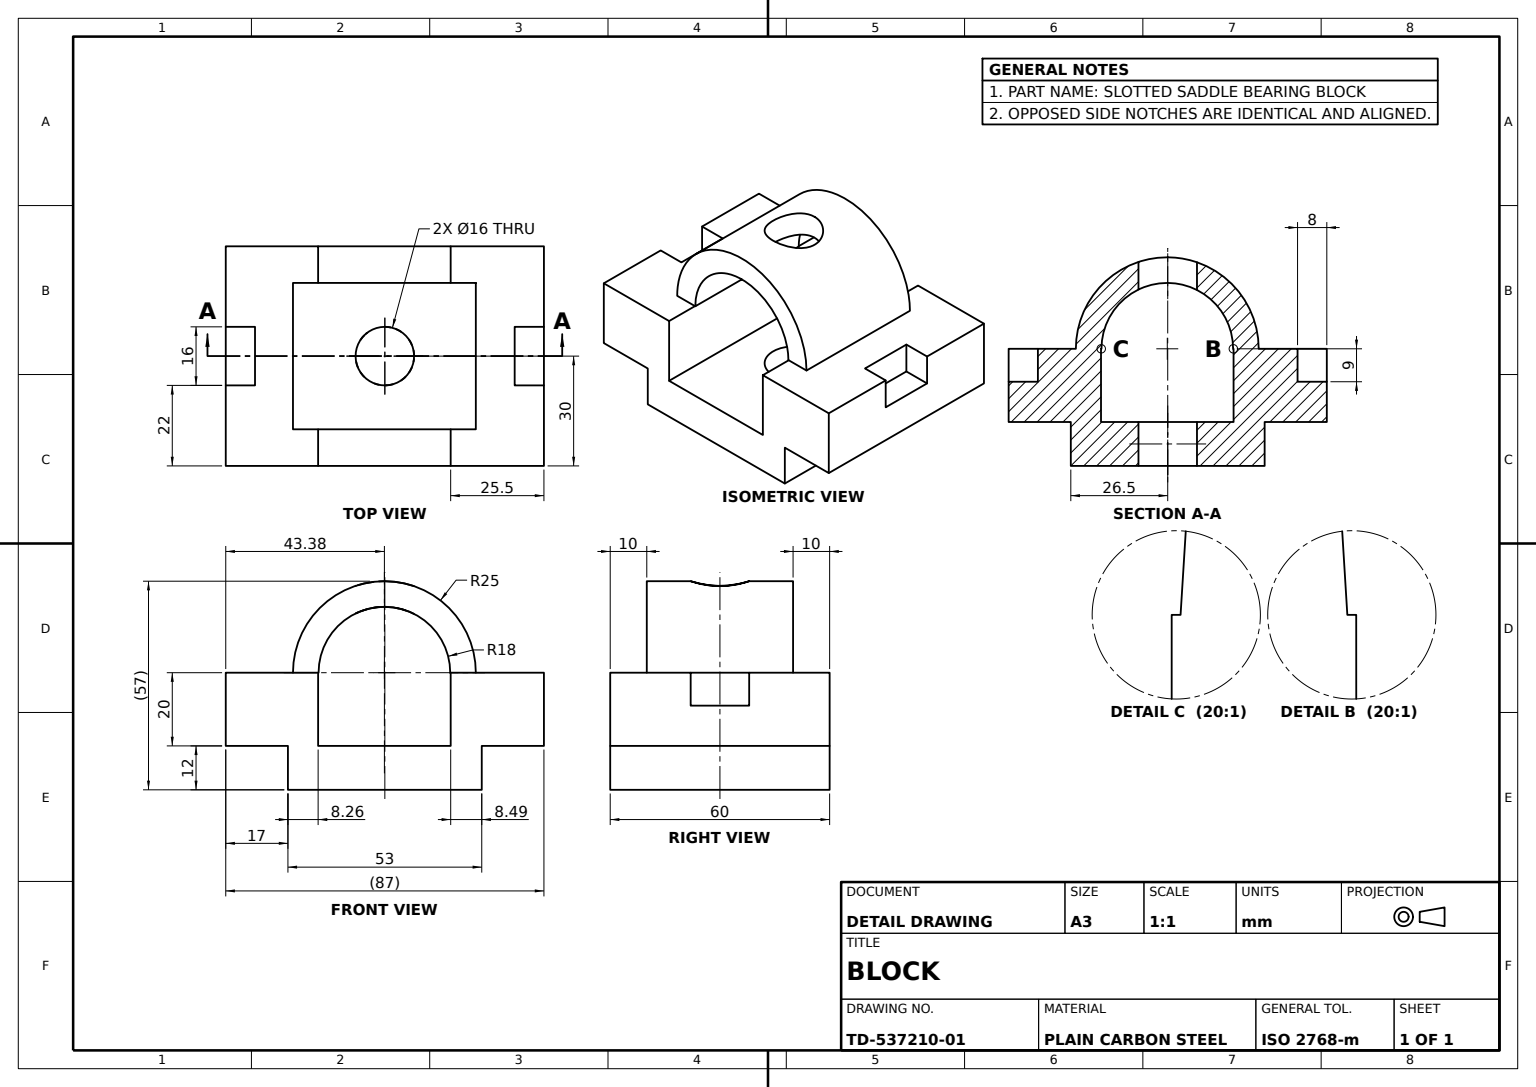
SolidWorks part; units mm, degrees
material "Plain Carbon Steel"
ref_plane "Front Plane" through (0, 0, 0) normal (0, 0, 1) x (1, 0, 0)
ref_plane "Top Plane" through (0, 0, 0) normal (0, 1, 0) x (1, 0, 0)
ref_plane "Right Plane" through (0, 0, 0) normal (1, 0, 0) x (0, 0, -1)
sketch "Base Block Profile" plane through (0, 0, 0) normal (0, 0, 1) x (1, 0, 0)
  line L0 (0, 0) -> (53, 0)
  line L1 (53, 0) -> (53, 12)
  line L2 (0, 0) -> (0, 12)
  line L3 (0, 12) -> (-17, 12)
  line L4 (53, 12) -> (70, 12)
  line L5 (-17, 12) -> (-17, 32)
  line L6 (-17, 32) -> (8.2571, 32)
  line L7 (70, 32) -> (70, 12)
  line L8 (8.2571, 32) -> (8.2571, 12)
  line L9 (8.2571, 12) -> (44.5084, 12)
  line L10 (44.5084, 12) -> (44.5, 32)
  line L11 (44.5, 32) -> (70, 32)
  dimension "D7" = 8.2571
  dimension "D1" = 53
  dimension "D2" = 12
  dimension "D3" = 12
  dimension "D4" = 17
  dimension "D5" = 17
  dimension "D6" = 20
  dimension "D8" = 8.4916
  dimension "D9" = 25.5
extrude "Base Block" add sketch "Base Block Profile" against normal blind 60
sketch "Saddle Arch Profile" plane through (0, 0, 0) normal (0, 0, 1) x (1, 0, 0)
  line L0 (8.2571, 32) -> (44.5, 32)
  line L1 (8.3786, 32) -> (1.3786, 32)
  line L2 (44.5, 32) -> (51.3786, 32)
  arc A0 (44.3786, 32) -> (8.3786, 32) centre (26.3786, 32) ccw
  arc A1 (51.3786, 32) -> (1.3786, 32) centre (26.3786, 32) ccw
  line M6 (70, 32) -> (44.5, 32)
  line M10 (8.2571, 32) -> (-17, 32)
  dimension "D1" = 18
  dimension "D2" = 25
extrude "Saddle Arch" add sketch "Saddle Arch Profile" against normal blind 60 contours A1 L0 A0 M6 M10
sketch "Bearing Seat Front Profile" plane through (0, 0, 0) normal (0, 0, 1) x (1, 0, 0)
  line L0 (8.2571, 32) -> (44.5, 32)
  line L1 (8.3786, 32) -> (1.3786, 32)
  line L2 (44.5, 32) -> (51.3786, 32)
  arc A0 (44.3786, 32) -> (8.3786, 32) centre (26.3786, 32) ccw
  arc A1 (51.3786, 32) -> (1.3786, 32) centre (26.3786, 32) ccw
  line M1 (44.3786, 32) -> (44.5, 32)
  line M5 (8.2571, 32) -> (8.3786, 32)
  arc M6 (8.3786, 32) -> (44.3786, 32) centre (26.3786, 32) cw
  arc M13 (51.3786, 32) -> (1.3786, 32) centre (26.3786, 32) ccw
  dimension "D1" = 18
extrude "Bearing Seat Cut Front" cut sketch "Bearing Seat Front Profile" against normal blind 10 contours L2 L1 M1 M13 M5 M6
sketch "Bearing Seat Rear Profile" plane through (0, 0, -60) normal (0, 0, -1) x (-1, 0, 0)
  line L0 (-51.3786, 32) -> (-44.3786, 32)
  line L1 (-8.3786, 32) -> (-1.3786, 32)
  arc A0 (-8.3786, 32) -> (-44.3786, 32) centre (-26.3786, 32) ccw
  arc A1 (-1.3786, 32) -> (-51.3786, 32) centre (-26.3786, 32) ccw
  dimension "D1" = 18
extrude "Bearing Seat Cut Rear" cut sketch "Bearing Seat Rear Profile" against normal blind 10
sketch "Oil Hole Sketch" plane through (0, 0, 0) normal (0, -1, 0) x (1, 0, 0)
  line L0 (0, -60) -> (0, 0) construction
  line L1 (0, 0) -> (53, 0) construction
  circle A0 centre (26.5, -30) radius 8
  dimension "D1" = 8
  dimension "D2" = 26.5
  dimension "D3" = 30
extrude "Oil Hole Ø8" cut sketch "Oil Hole Sketch" against normal blind 100
sketch "Locating Slots Sketch" plane through (0, 32, 0) normal (0, 1, 0) x (1, 0, 0)
  line L0 (-17, 38) -> (-17, 22)
  line L1 (-17, 60) -> (-17, 0) construction
  line L2 (-17, 38) -> (-9, 38)
  line L3 (-9, 38) -> (-9, 22)
  line L4 (-9, 22) -> (-17, 22)
  line L5 (8.2571, 60) -> (-17, 60) construction
  line L6 (70, 30) -> (70, 38)
  line L7 (70, 60) -> (70, 0) construction
  line L8 (70, 38) -> (62, 38)
  line L9 (62, 38) -> (62, 22)
  line L10 (62, 22) -> (70, 22)
  line L11 (70, 22) -> (70, 30)
  dimension "D1" = 22
  dimension "D2" = 8
  dimension "D3" = 16
  dimension "D4" = 8
  dimension "D5" = 8
  dimension "D6" = 16
extrude "Locating Slots" cut sketch "Locating Slots Sketch" against normal blind 9
